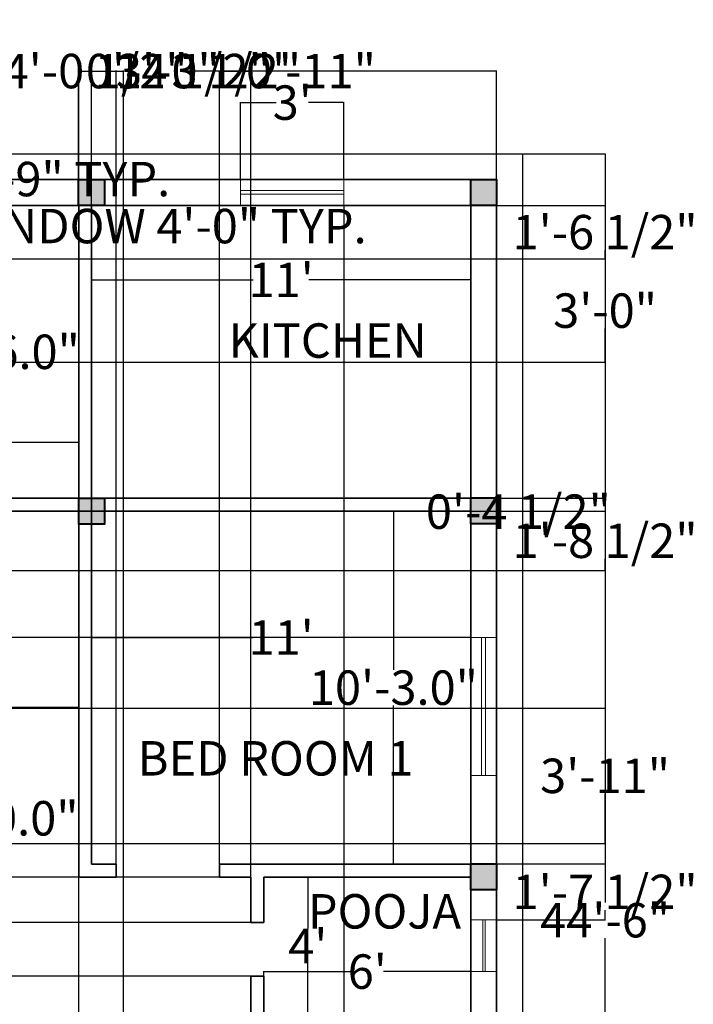
# Model space of a CAD drawing. Units: inches. Extents: x -132 to 363, y -548 to 79.
# Tile 3 of 3: x 128 to 363, y -264 to 79. Entities that reach past the tile are written whole.
import ezdxf

# ---------------------------------------------------------------- set-up
doc = ezdxf.new("R2010")
doc.units = ezdxf.units.IN
doc.header["$MEASUREMENT"] = 0
for name, color, linetype, lineweight in [('A-ANNO-DIMS', 2, 'Continuous', 18), ('A-AREA-IDEN', 7, 'Continuous', 25), ('A-COLS', 7, 'Continuous', 40), ('A-COLS-PATT', 252, 'Continuous', 13), ('A-GLAZ', 4, 'Continuous', 18), ('A-WALL', 7, 'Continuous', 35), ('C-PROP', 8, 'Continuous', 25)]:
    doc.layers.add(name, color=color, linetype=linetype, lineweight=lineweight)
doc.styles.get("Standard").update_dxf_attribs({"font": 'arial.ttf'})
doc.dimstyles.get("Standard").update_dxf_attribs({"dimtxt": 12, "dimasz": 0.18, "dimexe": 0.18, "dimexo": 0.0625, "dimgap": 0.09, "dimtad": 0, "dimtih": 1, "dimtoh": 1, "dimdec": 1, "dimzin": 0, "dimdsep": 46, "dimlunit": 3, "dimtxsty": 'Standard', "dimcen": 0.09, "dimadec": 0, "dimazin": 0, "dimtfac": 1, "dimtdec": 1, "dimtofl": 0, "dimtmove": 0, "dimatfit": 3, "dimfxl": 1, "dimtolj": 1, "dimtzin": 0, "dimarcsym": 0})

# ---------------------------------------------------------------- blocks, each defined once
blk = doc.blocks.new('*D1')
at = {"layer": 'A-ANNO-DIMS', "color": 0, "lineweight": -2, "transparency": 16777216}
for p, q in [((14.42, -87.55), (14.42, -68.07)), ((14.6, -68.25), (54.36, -68.25)), ((148.38, -68.25), (108.61, -68.25)), ((148.56, -87.55), (148.56, -68.07))]:
    blk.add_line(p, q, dxfattribs=at)
at = {"layer": 'A-ANNO-DIMS', "color": 0, "transparency": 16777216}
for points in [[(14.6, -68.22), (14.6, -68.28), (14.42, -68.25)], [(148.38, -68.22), (148.38, -68.28), (148.56, -68.25)]]:
    blk.add_solid(points, dxfattribs=at)
at = {"layer": 'Defpoints', "color": 0, "transparency": 16777216}
for p in [(148.56, -68.25), (14.42, -87.61), (148.56, -87.61)]:
    blk.add_point(p, dxfattribs=at)
at = {"layer": 'A-ANNO-DIMS', "color": 0, "transparency": 16777216, "insert": (81.49, -68.25), "char_height": 12, "attachment_point": 5}
blk.add_mtext('\\A1;11\'-2.1"', dxfattribs=at)
blk = doc.blocks.new('*D2')
at = {"layer": 'A-ANNO-DIMS', "color": 0, "lineweight": -2, "transparency": 16777216}
for p, q in [((148.4, 14.39), (123.86, 14.39)), ((124.04, 14.21), (124.04, -30.39)), ((124.04, -87.43), (124.04, -42.82)), ((148.45, -87.61), (123.86, -87.61))]:
    blk.add_line(p, q, dxfattribs=at)
at = {"layer": 'A-ANNO-DIMS', "color": 0, "transparency": 16777216}
for points in [[(124.01, 14.21), (124.07, 14.21), (124.04, 14.39)], [(124.01, -87.43), (124.07, -87.43), (124.04, -87.61)]]:
    blk.add_solid(points, dxfattribs=at)
at = {"layer": 'Defpoints', "color": 0, "transparency": 16777216}
for p in [(124.04, 14.39), (148.46, 14.39), (148.52, -87.61)]:
    blk.add_point(p, dxfattribs=at)
at = {"layer": 'A-ANNO-DIMS', "color": 0, "transparency": 16777216, "insert": (124.04, -36.61), "char_height": 12, "attachment_point": 5}
blk.add_mtext('\\A1;8\'-6.0"', dxfattribs=at)
blk = doc.blocks.new('*D3')
at = {"layer": 'A-ANNO-DIMS', "color": 0, "lineweight": -2, "transparency": 16777216}
for p, q in [((153.02, 14.33), (153.02, -11.75)), ((285.02, 14.33), (285.02, -11.75)), ((153.2, -11.57), (209.31, -11.57)), ((284.84, -11.57), (228.72, -11.57))]:
    blk.add_line(p, q, dxfattribs=at)
at = {"layer": 'A-ANNO-DIMS', "color": 0, "transparency": 16777216}
for points in [[(153.2, -11.54), (153.2, -11.6), (153.02, -11.57)], [(284.84, -11.54), (284.84, -11.6), (285.02, -11.57)]]:
    blk.add_solid(points, dxfattribs=at)
at = {"layer": 'Defpoints', "color": 0, "transparency": 16777216}
for p in [(153.02, 14.39), (285.02, 14.39), (285.02, -11.57)]:
    blk.add_point(p, dxfattribs=at)
at = {"layer": 'A-ANNO-DIMS', "color": 0, "transparency": 16777216, "insert": (219.02, -11.57), "char_height": 12, "attachment_point": 5}
blk.add_mtext("\\A1;11'", dxfattribs=at)
blk = doc.blocks.new('*D4')
at = {"layer": 'A-ANNO-DIMS', "color": 0, "lineweight": -2, "transparency": 16777216}
for p, q in [((284.95, -92.11), (257.94, -92.11)), ((258.12, -92.29), (258.12, -147.39)), ((258.12, -214.93), (258.12, -159.83)), ((284.95, -215.11), (257.94, -215.11))]:
    blk.add_line(p, q, dxfattribs=at)
at = {"layer": 'A-ANNO-DIMS', "color": 0, "transparency": 16777216}
for points in [[(258.09, -92.29), (258.15, -92.29), (258.12, -92.11)], [(258.09, -214.93), (258.15, -214.93), (258.12, -215.11)]]:
    blk.add_solid(points, dxfattribs=at)
at = {"layer": 'Defpoints', "color": 0, "transparency": 16777216}
for p in [(285.02, -92.11), (258.12, -215.11), (285.02, -215.11)]:
    blk.add_point(p, dxfattribs=at)
at = {"layer": 'A-ANNO-DIMS', "color": 0, "transparency": 16777216, "insert": (258.12, -153.61), "char_height": 12, "attachment_point": 5}
blk.add_mtext('\\A1;10\'-3.0"', dxfattribs=at)
blk = doc.blocks.new('*D5')
at = {"layer": 'A-ANNO-DIMS', "color": 0, "lineweight": -2, "transparency": 16777216}
for p, q in [((153.02, -134.95), (153.02, -136.33)), ((153.2, -136.15), (209.31, -136.15)), ((284.84, -136.15), (228.72, -136.15)), ((285.02, -136.09), (285.02, -135.97))]:
    blk.add_line(p, q, dxfattribs=at)
at = {"layer": 'A-ANNO-DIMS', "color": 0, "transparency": 16777216}
for points in [[(153.2, -136.12), (153.2, -136.18), (153.02, -136.15)], [(284.84, -136.12), (284.84, -136.18), (285.02, -136.15)]]:
    blk.add_solid(points, dxfattribs=at)
at = {"layer": 'Defpoints', "color": 0, "transparency": 16777216}
for p in [(153.02, -134.89), (285.02, -136.15), (285.02, -136.15)]:
    blk.add_point(p, dxfattribs=at)
at = {"layer": 'A-ANNO-DIMS', "color": 0, "transparency": 16777216, "insert": (219.02, -136.15), "char_height": 12, "attachment_point": 5}
blk.add_mtext("\\A1;11'", dxfattribs=at)
blk = doc.blocks.new('*D6')
at = {"layer": 'A-ANNO-DIMS', "color": 0, "lineweight": -2, "transparency": 16777216}
for p, q in [((213.08, -219.61), (228.48, -219.61)), ((228.3, -219.79), (228.3, -237.52)), ((228.3, -267.43), (228.3, -249.7)), ((213.08, -267.61), (228.48, -267.61))]:
    blk.add_line(p, q, dxfattribs=at)
at = {"layer": 'A-ANNO-DIMS', "color": 0, "transparency": 16777216}
for points in [[(228.27, -219.79), (228.33, -219.79), (228.3, -219.61)], [(228.27, -267.43), (228.33, -267.43), (228.3, -267.61)]]:
    blk.add_solid(points, dxfattribs=at)
at = {"layer": 'Defpoints', "color": 0, "transparency": 16777216}
for p in [(213.02, -219.61), (213.02, -267.61), (228.3, -267.61)]:
    blk.add_point(p, dxfattribs=at)
at = {"layer": 'A-ANNO-DIMS', "color": 0, "transparency": 16777216, "insert": (228.3, -243.61), "char_height": 12, "attachment_point": 5}
blk.add_mtext("\\A1;4'", dxfattribs=at)
blk = doc.blocks.new('*D7')
at = {"layer": 'A-ANNO-DIMS', "color": 0, "lineweight": -2, "transparency": 16777216}
for p, q in [((213.02, -254.06), (213.02, -252.33)), ((213.2, -252.51), (243.37, -252.51)), ((284.84, -252.51), (254.66, -252.51)), ((285.02, -252.45), (285.02, -252.33))]:
    blk.add_line(p, q, dxfattribs=at)
at = {"layer": 'A-ANNO-DIMS', "color": 0, "transparency": 16777216}
for points in [[(213.2, -252.48), (213.2, -252.54), (213.02, -252.51)], [(284.84, -252.48), (284.84, -252.54), (285.02, -252.51)]]:
    blk.add_solid(points, dxfattribs=at)
at = {"layer": 'Defpoints', "color": 0, "transparency": 16777216}
for p in [(285.02, -252.51), (285.02, -252.51), (213.02, -254.12)]:
    blk.add_point(p, dxfattribs=at)
at = {"layer": 'A-ANNO-DIMS', "color": 0, "transparency": 16777216, "insert": (249.02, -252.51), "char_height": 12, "attachment_point": 5}
blk.add_mtext("\\A1;6'", dxfattribs=at)
blk = doc.blocks.new('*D15')
at = {"layer": 'A-ANNO-DIMS', "color": 0, "lineweight": -2, "transparency": 16777216}
for p, q in [((14.42, -160.68), (14.42, -160.33)), ((14.6, -160.51), (54.34, -160.51)), ((148.34, -160.51), (108.59, -160.51)), ((148.52, -160.68), (148.52, -160.33))]:
    blk.add_line(p, q, dxfattribs=at)
at = {"layer": 'A-ANNO-DIMS', "color": 0, "transparency": 16777216}
for points in [[(14.6, -160.48), (14.6, -160.54), (14.42, -160.51)], [(148.34, -160.48), (148.34, -160.54), (148.52, -160.51)]]:
    blk.add_solid(points, dxfattribs=at)
at = {"layer": 'Defpoints', "color": 0, "transparency": 16777216}
for p in [(14.42, -160.75), (148.52, -160.51), (148.52, -160.75)]:
    blk.add_point(p, dxfattribs=at)
at = {"layer": 'A-ANNO-DIMS', "color": 0, "transparency": 16777216, "insert": (81.47, -160.51), "char_height": 12, "attachment_point": 5}
blk.add_mtext('\\A1;11\'-2.1"', dxfattribs=at)
blk = doc.blocks.new('*D16')
at = {"layer": 'A-ANNO-DIMS', "color": 0, "lineweight": -2, "transparency": 16777216}
for p, q in [((148.45, -92.11), (114.32, -92.11)), ((114.5, -92.29), (114.5, -192.89)), ((114.5, -305.93), (114.5, -205.32)), ((148.45, -306.11), (114.32, -306.11))]:
    blk.add_line(p, q, dxfattribs=at)
at = {"layer": 'A-ANNO-DIMS', "color": 0, "transparency": 16777216}
for points in [[(114.47, -92.29), (114.53, -92.29), (114.5, -92.11)], [(114.47, -305.93), (114.53, -305.93), (114.5, -306.11)]]:
    blk.add_solid(points, dxfattribs=at)
at = {"layer": 'Defpoints', "color": 0, "transparency": 16777216}
for p in [(148.52, -92.11), (114.5, -306.11), (148.52, -306.11)]:
    blk.add_point(p, dxfattribs=at)
at = {"layer": 'A-ANNO-DIMS', "color": 0, "transparency": 16777216, "insert": (114.5, -199.11), "char_height": 12, "attachment_point": 5}
blk.add_mtext('\\A1;17\'-10.0"', dxfattribs=at)
blk = doc.blocks.new('*D18')
at = {"layer": 'A-ANNO-DIMS', "color": 0, "lineweight": -2, "transparency": 16777216}
for p, q in [((204.9, 23.45), (204.9, 50.38)), ((205.08, 50.2), (217.3, 50.2)), ((240.72, 50.2), (228.51, 50.2)), ((240.9, 23.45), (240.9, 50.38))]:
    blk.add_line(p, q, dxfattribs=at)
at = {"layer": 'A-ANNO-DIMS', "color": 0, "transparency": 16777216}
for points in [[(205.08, 50.23), (205.08, 50.17), (204.9, 50.2)], [(240.72, 50.23), (240.72, 50.17), (240.9, 50.2)]]:
    blk.add_solid(points, dxfattribs=at)
at = {"layer": 'Defpoints', "color": 0, "transparency": 16777216}
for p in [(240.9, 50.2), (204.9, 23.39), (240.9, 23.39)]:
    blk.add_point(p, dxfattribs=at)
at = {"layer": 'A-ANNO-DIMS', "color": 0, "transparency": 16777216, "insert": (222.9, 50.2), "char_height": 12, "attachment_point": 5}
blk.add_mtext("\\A1;3'", dxfattribs=at)
blk = doc.blocks.new('WIN-48IN')
for p, q in [((48, 9), (0, 9)), ((0, 9), (0, 0)), ((48, 0), (48, 9)), ((0, 5.12), (48, 5.12)), ((48, 5.12), (0, 5.12)), ((0, 3.8), (48, 3.8)), ((0, 0), (48, 0))]:
    blk.add_line(p, q)
blk = doc.blocks.new('WIN-18IN')
for p, q in [((18, 9), (0, 9)), ((0, 9), (0, 0)), ((18, 0), (18, 9)), ((0, 6), (0, 0)), ((18, 5.06), (0, 5.06)), ((18, 4.2), (0, 4.2)), ((18, 0), (18, 6)), ((0, 0), (18, 0)), ((0, 0), (18, 0)), ((0, 0), (18, 0))]:
    blk.add_line(p, q)
blk = doc.blocks.new('*D21')
at = {"layer": 'A-ANNO-DIMS', "color": 0, "lineweight": -2, "transparency": 16777216}
for p, q in [((51.75, 14.33), (51.75, 7.01)), ((99.75, 14.33), (99.75, 7.01)), ((51.93, 7.19), (99.57, 7.19)), ((99.75, 7.19), (99.93, 7.19))]:
    blk.add_line(p, q, dxfattribs=at)
at = {"layer": 'A-ANNO-DIMS', "color": 0, "transparency": 16777216}
for points in [[(51.93, 7.22), (51.93, 7.16), (51.75, 7.19)], [(99.57, 7.22), (99.57, 7.16), (99.75, 7.19)]]:
    blk.add_solid(points, dxfattribs=at)
at = {"layer": 'Defpoints', "color": 0, "transparency": 16777216}
for p in [(51.75, 14.39), (99.75, 14.39), (99.75, 7.19)]:
    blk.add_point(p, dxfattribs=at)
at = {"layer": 'A-ANNO-DIMS', "color": 0, "transparency": 16777216, "insert": (175.94, 7.19), "char_height": 12, "attachment_point": 5}
blk.add_mtext('\\A1;WINDOW 4\'-0" TYP.', dxfattribs=at)
blk = doc.blocks.new('*D22')
at = {"layer": 'A-ANNO-DIMS', "color": 0, "lineweight": -2, "transparency": 16777216}
for p, q in [((99.81, 23.39), (107.13, 23.39)), ((106.95, 23.39), (106.95, 23.57)), ((106.95, 23.57), (107.13, 23.57)), ((106.95, 14.57), (106.95, 23.21)), ((99.81, 14.39), (107.13, 14.39))]:
    blk.add_line(p, q, dxfattribs=at)
at = {"layer": 'A-ANNO-DIMS', "color": 0, "transparency": 16777216}
for points in [[(106.92, 23.21), (106.98, 23.21), (106.95, 23.39)], [(106.92, 14.57), (106.98, 14.57), (106.95, 14.39)]]:
    blk.add_solid(points, dxfattribs=at)
at = {"layer": 'Defpoints', "color": 0, "transparency": 16777216}
for p in [(99.75, 23.39), (106.95, 23.39), (99.75, 14.39)]:
    blk.add_point(p, dxfattribs=at)
at = {"layer": 'A-ANNO-DIMS', "color": 0, "transparency": 16777216, "insert": (143.79, 23.57), "char_height": 12, "attachment_point": 5}
blk.add_mtext('\\A1;0\'-9" TYP.', dxfattribs=at)
blk = doc.blocks.new('*D26')
at = {"layer": 'A-ANNO-DIMS', "color": 0, "lineweight": -2, "transparency": 16777216}
for p, q in [((303.08, 32.39), (332, 32.39)), ((331.82, 32.21), (331.82, -228.39)), ((331.82, -501.43), (331.82, -240.82)), ((303.08, -501.61), (332, -501.61))]:
    blk.add_line(p, q, dxfattribs=at)
at = {"layer": 'A-ANNO-DIMS', "color": 0, "transparency": 16777216}
for points in [[(331.79, 32.21), (331.85, 32.21), (331.82, 32.39)], [(331.79, -501.43), (331.85, -501.43), (331.82, -501.61)]]:
    blk.add_solid(points, dxfattribs=at)
at = {"layer": 'Defpoints', "color": 0, "transparency": 16777216}
for p in [(303.02, 32.39), (303.02, -501.61), (331.82, -501.61)]:
    blk.add_point(p, dxfattribs=at)
at = {"layer": 'A-ANNO-DIMS', "color": 0, "transparency": 16777216, "insert": (331.82, -234.61), "char_height": 12, "attachment_point": 5}
blk.add_mtext('\\A1;44\'-6"', dxfattribs=at)
blk = doc.blocks.new('*D27')
at = {"layer": 'A-ANNO-DIMS', "color": 0, "lineweight": -2, "transparency": 16777216}
for p, q in [((5.42, 23.45), (5.42, 61.37)), ((5.6, 61.19), (114.93, 61.19)), ((293.84, 61.19), (184.5, 61.19)), ((294.02, 23.45), (294.02, 61.37))]:
    blk.add_line(p, q, dxfattribs=at)
at = {"layer": 'A-ANNO-DIMS', "color": 0, "transparency": 16777216}
for points in [[(5.6, 61.22), (5.6, 61.16), (5.42, 61.19)], [(293.84, 61.22), (293.84, 61.16), (294.02, 61.19)]]:
    blk.add_solid(points, dxfattribs=at)
at = {"layer": 'Defpoints', "color": 0, "transparency": 16777216}
for p in [(294.02, 61.19), (5.42, 23.39), (294.02, 23.39)]:
    blk.add_point(p, dxfattribs=at)
at = {"layer": 'A-ANNO-DIMS', "color": 0, "transparency": 16777216, "insert": (149.72, 61.19), "char_height": 12, "attachment_point": 5}
blk.add_mtext('\\A1;24\'-0 1/2"', dxfattribs=at)
blk = doc.blocks.new('*D30')
at = {"layer": 'A-ANNO-DIMS', "color": 0, "lineweight": -2, "transparency": 16777216}
for p, q in [((240.9, 14.33), (240.9, -530.59)), ((285.02, 14.33), (285.02, -530.59)), ((241.08, -530.41), (246.92, -530.41)), ((284.84, -530.41), (278.99, -530.41))]:
    blk.add_line(p, q, dxfattribs=at)
at = {"layer": 'A-ANNO-DIMS', "color": 0, "transparency": 16777216}
for points in [[(241.08, -530.38), (241.08, -530.44), (240.9, -530.41)], [(284.84, -530.38), (284.84, -530.44), (285.02, -530.41)]]:
    blk.add_solid(points, dxfattribs=at)
at = {"layer": 'Defpoints', "color": 0, "transparency": 16777216}
for p in [(240.9, 14.39), (285.02, 14.39), (285.02, -530.41)]:
    blk.add_point(p, dxfattribs=at)
at = {"layer": 'A-ANNO-DIMS', "color": 0, "transparency": 16777216, "insert": (262.96, -530.41), "char_height": 12, "attachment_point": 5}
blk.add_mtext('\\A1;3\'-8"', dxfattribs=at)
blk = doc.blocks.new('*D31')
at = {"layer": 'A-ANNO-DIMS', "color": 0, "lineweight": -2, "transparency": 16777216}
for p, q in [((14.48, 14.39), (332, 14.39)), ((331.82, 14.21), (331.82, 11.36)), ((331.82, -4.08), (331.82, -1.23)), ((14.48, -4.26), (332, -4.26))]:
    blk.add_line(p, q, dxfattribs=at)
at = {"layer": 'A-ANNO-DIMS', "color": 0, "transparency": 16777216}
for points in [[(331.79, 14.21), (331.85, 14.21), (331.82, 14.39)], [(331.79, -4.08), (331.85, -4.08), (331.82, -4.26)]]:
    blk.add_solid(points, dxfattribs=at)
at = {"layer": 'Defpoints', "color": 0, "transparency": 16777216}
for p in [(14.42, 14.39), (14.42, -4.26), (331.82, -4.26)]:
    blk.add_point(p, dxfattribs=at)
at = {"layer": 'A-ANNO-DIMS', "color": 0, "transparency": 16777216, "insert": (331.82, 5.07), "char_height": 12, "attachment_point": 5}
blk.add_mtext('\\A1;1\'-6 1/2"', dxfattribs=at)
blk = doc.blocks.new('*D32')
at = {"layer": 'A-ANNO-DIMS', "color": 0, "lineweight": -2, "transparency": 16777216}
for p, q in [((14.48, -4.26), (332, -4.26)), ((331.82, -4.44), (331.82, -16.04)), ((331.82, -40.08), (331.82, -28.48)), ((14.48, -40.26), (332, -40.26))]:
    blk.add_line(p, q, dxfattribs=at)
at = {"layer": 'A-ANNO-DIMS', "color": 0, "transparency": 16777216}
for points in [[(331.79, -4.44), (331.85, -4.44), (331.82, -4.26)], [(331.79, -40.08), (331.85, -40.08), (331.82, -40.26)]]:
    blk.add_solid(points, dxfattribs=at)
at = {"layer": 'Defpoints', "color": 0, "transparency": 16777216}
for p in [(14.42, -4.26), (14.42, -40.26), (331.82, -40.26)]:
    blk.add_point(p, dxfattribs=at)
at = {"layer": 'A-ANNO-DIMS', "color": 0, "transparency": 16777216, "insert": (331.82, -22.26), "char_height": 12, "attachment_point": 5}
blk.add_mtext('\\A1;3\'-0"', dxfattribs=at)
blk = doc.blocks.new('*D33')
at = {"layer": 'A-ANNO-DIMS', "color": 0, "lineweight": -2, "transparency": 16777216}
for p, q in [((14.48, -92.11), (332, -92.11)), ((331.82, -92.29), (331.82, -96.13)), ((331.82, -112.57), (331.82, -108.72)), ((14.48, -112.75), (332, -112.75))]:
    blk.add_line(p, q, dxfattribs=at)
at = {"layer": 'A-ANNO-DIMS', "color": 0, "transparency": 16777216}
for points in [[(331.79, -92.29), (331.85, -92.29), (331.82, -92.11)], [(331.79, -112.57), (331.85, -112.57), (331.82, -112.75)]]:
    blk.add_solid(points, dxfattribs=at)
at = {"layer": 'Defpoints', "color": 0, "transparency": 16777216}
for p in [(14.42, -92.11), (14.42, -112.75), (331.82, -112.75)]:
    blk.add_point(p, dxfattribs=at)
at = {"layer": 'A-ANNO-DIMS', "color": 0, "transparency": 16777216, "insert": (331.82, -102.43), "char_height": 12, "attachment_point": 5}
blk.add_mtext('\\A1;1\'-8 1/2"', dxfattribs=at)
blk = doc.blocks.new('*D34')
at = {"layer": 'A-ANNO-DIMS', "color": 0, "lineweight": -2, "transparency": 16777216}
for p, q in [((14.48, -160.75), (332, -160.75)), ((331.82, -160.93), (331.82, -178.11)), ((331.82, -207.73), (331.82, -190.55)), ((14.48, -207.91), (332, -207.91))]:
    blk.add_line(p, q, dxfattribs=at)
at = {"layer": 'A-ANNO-DIMS', "color": 0, "transparency": 16777216}
for points in [[(331.79, -160.93), (331.85, -160.93), (331.82, -160.75)], [(331.79, -207.73), (331.85, -207.73), (331.82, -207.91)]]:
    blk.add_solid(points, dxfattribs=at)
at = {"layer": 'Defpoints', "color": 0, "transparency": 16777216}
for p in [(14.42, -160.75), (14.42, -207.91), (331.82, -207.91)]:
    blk.add_point(p, dxfattribs=at)
at = {"layer": 'A-ANNO-DIMS', "color": 0, "transparency": 16777216, "insert": (331.82, -184.33), "char_height": 12, "attachment_point": 5}
blk.add_mtext('\\A1;3\'-11"', dxfattribs=at)
blk = doc.blocks.new('*D35')
at = {"layer": 'A-ANNO-DIMS', "color": 0, "lineweight": -2, "transparency": 16777216}
for p, q in [((284.95, -92.11), (-70.46, -92.11)), ((-70.28, -92.29), (-70.28, -107.91)), ((-70.28, -135.97), (-70.28, -120.35)), ((284.95, -136.15), (-70.46, -136.15))]:
    blk.add_line(p, q, dxfattribs=at)
at = {"layer": 'A-ANNO-DIMS', "color": 0, "transparency": 16777216}
for points in [[(-70.31, -92.29), (-70.25, -92.29), (-70.28, -92.11)], [(-70.31, -135.97), (-70.25, -135.97), (-70.28, -136.15)]]:
    blk.add_solid(points, dxfattribs=at)
at = {"layer": 'Defpoints', "color": 0, "transparency": 16777216}
for p in [(285.02, -92.11), (-70.28, -136.15), (285.02, -136.15)]:
    blk.add_point(p, dxfattribs=at)
at = {"layer": 'A-ANNO-DIMS', "color": 0, "transparency": 16777216, "insert": (-70.28, -114.13), "char_height": 12, "attachment_point": 5}
blk.add_mtext('\\A1;3\'-8"', dxfattribs=at)
blk = doc.blocks.new('*D36')
at = {"layer": 'A-ANNO-DIMS', "color": 0, "lineweight": -2, "transparency": 16777216}
for p, q in [((294.08, -215.01), (332, -215.01)), ((331.82, -215.19), (331.82, -218.47)), ((331.82, -234.33), (331.82, -231.06)), ((294.08, -234.51), (332, -234.51))]:
    blk.add_line(p, q, dxfattribs=at)
at = {"layer": 'A-ANNO-DIMS', "color": 0, "transparency": 16777216}
for points in [[(331.79, -215.19), (331.85, -215.19), (331.82, -215.01)], [(331.79, -234.33), (331.85, -234.33), (331.82, -234.51)]]:
    blk.add_solid(points, dxfattribs=at)
at = {"layer": 'Defpoints', "color": 0, "transparency": 16777216}
for p in [(294.02, -215.01), (294.02, -234.51), (331.82, -234.51)]:
    blk.add_point(p, dxfattribs=at)
at = {"layer": 'A-ANNO-DIMS', "color": 0, "transparency": 16777216, "insert": (331.82, -224.76), "char_height": 12, "attachment_point": 5}
blk.add_mtext('\\A1;1\'-7 1/2"', dxfattribs=at)
blk = doc.blocks.new('*D44')
at = {"layer": 'A-ANNO-DIMS', "color": 0, "lineweight": -2, "transparency": 16777216}
for p, q in [((161.59, -215.05), (161.59, 61.37)), ((161.77, 61.19), (163.55, 61.19)), ((197.41, 61.19), (195.62, 61.19)), ((197.59, -215.05), (197.59, 61.37))]:
    blk.add_line(p, q, dxfattribs=at)
at = {"layer": 'A-ANNO-DIMS', "color": 0, "transparency": 16777216}
for points in [[(161.77, 61.22), (161.77, 61.16), (161.59, 61.19)], [(197.41, 61.22), (197.41, 61.16), (197.59, 61.19)]]:
    blk.add_solid(points, dxfattribs=at)
at = {"layer": 'Defpoints', "color": 0, "transparency": 16777216}
for p in [(197.59, 61.19), (161.59, -215.11), (197.59, -215.11)]:
    blk.add_point(p, dxfattribs=at)
at = {"layer": 'A-ANNO-DIMS', "color": 0, "transparency": 16777216, "insert": (179.59, 61.19), "char_height": 12, "attachment_point": 5}
blk.add_mtext('\\A1;3\'-0"', dxfattribs=at)
blk = doc.blocks.new('*D46')
at = {"layer": 'A-ANNO-DIMS', "color": 0, "lineweight": -2, "transparency": 16777216}
for p, q in [((208.45, -235.36), (-70.46, -235.36)), ((-70.28, -235.54), (-70.28, -238.62)), ((-70.28, -253.94), (-70.28, -250.85)), ((208.45, -254.12), (-70.46, -254.12))]:
    blk.add_line(p, q, dxfattribs=at)
at = {"layer": 'A-ANNO-DIMS', "color": 0, "transparency": 16777216}
for points in [[(-70.31, -235.54), (-70.25, -235.54), (-70.28, -235.36)], [(-70.31, -253.94), (-70.25, -253.94), (-70.28, -254.12)]]:
    blk.add_solid(points, dxfattribs=at)
at = {"layer": 'Defpoints', "color": 0, "transparency": 16777216}
for p in [(208.52, -235.36), (-70.28, -254.12), (208.52, -254.12)]:
    blk.add_point(p, dxfattribs=at)
at = {"layer": 'A-ANNO-DIMS', "color": 0, "transparency": 16777216, "insert": (-70.28, -244.74), "char_height": 12, "attachment_point": 5}
blk.add_mtext('\\A1;1\'-7"', dxfattribs=at)
blk = doc.blocks.new('*D48')
at = {"layer": 'A-ANNO-DIMS', "color": 0, "lineweight": -2, "transparency": 16777216}
for p, q in [((197.59, -219.55), (197.59, 61.37)), ((197.77, 61.19), (208.34, 61.19)), ((208.52, -219.55), (208.52, 61.37)), ((208.52, 61.19), (208.7, 61.19))]:
    blk.add_line(p, q, dxfattribs=at)
at = {"layer": 'A-ANNO-DIMS', "color": 0, "transparency": 16777216}
for points in [[(197.77, 61.22), (197.77, 61.16), (197.59, 61.19)], [(208.34, 61.22), (208.34, 61.16), (208.52, 61.19)]]:
    blk.add_solid(points, dxfattribs=at)
at = {"layer": 'Defpoints', "color": 0, "transparency": 16777216}
for p in [(208.52, 61.19), (197.59, -219.61), (208.52, -219.61)]:
    blk.add_point(p, dxfattribs=at)
at = {"layer": 'A-ANNO-DIMS', "color": 0, "transparency": 16777216, "insert": (229.4, 61.19), "char_height": 12, "attachment_point": 5}
blk.add_mtext('\\A1;0\'-11"', dxfattribs=at)
blk = doc.blocks.new('*D50')
at = {"layer": 'A-ANNO-DIMS', "color": 0, "lineweight": -2, "transparency": 16777216}
for p, q in [((208.45, -219.61), (-70.46, -219.61)), ((-70.28, -219.79), (-70.28, -221.37)), ((208.45, -235.36), (-70.46, -235.36)), ((-70.28, -235.18), (-70.28, -233.6))]:
    blk.add_line(p, q, dxfattribs=at)
at = {"layer": 'A-ANNO-DIMS', "color": 0, "transparency": 16777216}
for points in [[(-70.31, -219.79), (-70.25, -219.79), (-70.28, -219.61)], [(-70.31, -235.18), (-70.25, -235.18), (-70.28, -235.36)]]:
    blk.add_solid(points, dxfattribs=at)
at = {"layer": 'Defpoints', "color": 0, "transparency": 16777216}
for p in [(208.52, -219.61), (-70.28, -235.36), (208.52, -235.36)]:
    blk.add_point(p, dxfattribs=at)
at = {"layer": 'A-ANNO-DIMS', "color": 0, "transparency": 16777216, "insert": (-70.28, -227.48), "char_height": 12, "attachment_point": 5}
blk.add_mtext('\\A1;1\'-4"', dxfattribs=at)
blk = doc.blocks.new('*D52')
at = {"layer": 'A-ANNO-DIMS', "color": 0, "lineweight": -2, "transparency": 16777216}
for p, q in [((148.46, 14.45), (148.46, 61.37)), ((148.64, 61.19), (152.84, 61.19)), ((153.02, 14.45), (153.02, 61.37)), ((153.02, 61.19), (153.2, 61.19))]:
    blk.add_line(p, q, dxfattribs=at)
at = {"layer": 'A-ANNO-DIMS', "color": 0, "transparency": 16777216}
for points in [[(148.64, 61.22), (148.64, 61.16), (148.46, 61.19)], [(152.84, 61.22), (152.84, 61.16), (153.02, 61.19)]]:
    blk.add_solid(points, dxfattribs=at)
at = {"layer": 'Defpoints', "color": 0, "transparency": 16777216}
for p in [(153.02, 61.19), (148.46, 14.39), (153.02, 14.39)]:
    blk.add_point(p, dxfattribs=at)
at = {"layer": 'A-ANNO-DIMS', "color": 0, "transparency": 16777216, "insert": (183.22, 61.19), "char_height": 12, "attachment_point": 5}
blk.add_mtext('\\A1;0\'-4 1/2"', dxfattribs=at)
blk = doc.blocks.new('*D57')
at = {"layer": 'A-ANNO-DIMS', "color": 0, "lineweight": -2, "transparency": 16777216}
for p, q in [((148.52, -267.55), (148.52, 61.37)), ((148.7, 61.19), (163.91, 61.19)), ((164.09, -267.55), (164.09, 61.37)), ((164.09, 61.19), (164.27, 61.19))]:
    blk.add_line(p, q, dxfattribs=at)
at = {"layer": 'A-ANNO-DIMS', "color": 0, "transparency": 16777216}
for points in [[(148.7, 61.22), (148.7, 61.16), (148.52, 61.19)], [(163.91, 61.22), (163.91, 61.16), (164.09, 61.19)]]:
    blk.add_solid(points, dxfattribs=at)
at = {"layer": 'Defpoints', "color": 0, "transparency": 16777216}
for p in [(164.09, 61.19), (148.52, -267.61), (164.09, -267.61)]:
    blk.add_point(p, dxfattribs=at)
at = {"layer": 'A-ANNO-DIMS', "color": 0, "transparency": 16777216, "insert": (193.73, 61.19), "char_height": 12, "attachment_point": 5}
blk.add_mtext('\\A1;1\'-3 1/2"', dxfattribs=at)
blk = doc.blocks.new('*D58')
at = {"layer": 'A-ANNO-DIMS', "color": 0, "lineweight": -2, "transparency": 16777216}
for p, q in [((285.08, -87.61), (332, -87.61)), ((331.82, -87.79), (331.82, -91.93)), ((285.08, -92.11), (332, -92.11)), ((331.82, -92.29), (331.64, -92.29)), ((331.82, -92.11), (331.82, -92.29))]:
    blk.add_line(p, q, dxfattribs=at)
at = {"layer": 'A-ANNO-DIMS', "color": 0, "transparency": 16777216}
for points in [[(331.79, -87.79), (331.85, -87.79), (331.82, -87.61)], [(331.79, -91.93), (331.85, -91.93), (331.82, -92.11)]]:
    blk.add_solid(points, dxfattribs=at)
at = {"layer": 'Defpoints', "color": 0, "transparency": 16777216}
for p in [(285.02, -87.61), (285.02, -92.11), (331.82, -92.11)]:
    blk.add_point(p, dxfattribs=at)
at = {"layer": 'A-ANNO-DIMS', "color": 0, "transparency": 16777216, "insert": (301.62, -92.29), "char_height": 12, "attachment_point": 5}
blk.add_mtext('\\A1;0\'-4 1/2"', dxfattribs=at)

msp = doc.modelspace()

# ---------------------------------------------------------------- hatches: boundary and pattern name
at = {"layer": 'A-COLS-PATT'}
h = msp.add_hatch(color=256, dxfattribs=at)
h.dxf.hatch_style = 1
h.paths.add_polyline_path([(14.42, 23.39), (6.02, 23.39), (5.42, 23.39), (5.42, 14.39), (14.42, 14.39)])
h.paths.add_polyline_path([(14.42, -87.61), (5.42, -87.61), (5.42, -96.61), (14.42, -96.61)])
h.paths.add_polyline_path([(153.02, -87.61), (148.56, -87.61), (148.56, -96.61), (153.02, -96.61)])
h.paths.add_polyline_path([(157.56, -87.61), (153.02, -87.61), (153.02, -92.11), (157.56, -92.11)])
h.paths.add_polyline_path([(157.56, -92.11), (153.02, -92.11), (153.02, -96.61), (157.56, -96.61)])
h.paths.add_polyline_path([(294.02, -87.49), (285.02, -87.49), (285.02, -96.49), (294.02, -96.49)])
h.paths.add_polyline_path([(294.02, -215.01), (285.02, -215.01), (285.02, -224.01), (294.02, -224.01)])
h.paths.add_polyline_path([(294.02, -267.43), (285.02, -267.43), (285.02, -277.01), (294.02, -277.01)])
h.paths.add_polyline_path([(294.02, -406.11), (285.02, -406.11), (285.02, -415.11), (294.02, -415.11)])
h.paths.add_polyline_path([(161.71, -406.11), (148.52, -406.11), (148.52, -415.11), (161.71, -415.11)])
h.paths.add_polyline_path([(157.51, -267.61), (148.52, -267.61), (148.52, -276.61), (157.51, -276.61)])
h.paths.add_polyline_path([(14.42, -268.43), (5.42, -268.43), (5.42, -277.43), (14.42, -277.43)])
h = msp.add_hatch(color=256, dxfattribs=at)
h.dxf.hatch_style = 1
h.paths.add_polyline_path([(294.02, 23.39), (285.02, 23.39), (285.02, 14.39), (294.02, 14.39)])
h.paths.add_polyline_path([(157.46, 23.39), (148.46, 23.39), (148.46, 14.39), (157.46, 14.39)])
h = msp.add_hatch(color=256, dxfattribs=at)
h.dxf.hatch_style = 1
h.paths.add_polyline_path([(285.02, 23.39), (285.02, 14.39), (294.02, 14.39), (294.02, 23.39)])
h.paths.add_polyline_path([(148.46, 23.39), (148.46, 14.39), (157.46, 14.39), (157.46, 23.39)])

# ---------------------------------------------------------------- linework, layer by layer
at = {"layer": 'A-COLS'}
for points in [[(148.46, 23.39), (157.46, 23.39), (157.46, 14.39), (148.46, 14.39)], [(285.02, 23.39), (294.02, 23.39), (294.02, 14.39), (285.02, 14.39)], [(148.56, -87.61), (157.56, -87.61), (157.56, -96.61), (148.56, -96.61)], [(285.02, -87.49), (294.02, -87.49), (294.02, -96.49), (285.02, -96.49)], [(285.02, -215.01), (294.02, -215.01), (294.02, -224.01), (285.02, -224.01)]]:
    msp.add_lwpolyline(points, close=True, dxfattribs=at)
at = {"layer": 'A-GLAZ'}
for p, q in [((240.9, 23.39), (204.9, 23.39)), ((204.9, 23.39), (204.9, 14.39)), ((240.9, 14.39), (240.9, 23.39)), ((240.9, 19.59), (204.9, 19.59)), ((240.9, 18.28), (204.9, 18.28)), ((204.9, 18.28), (240.9, 18.28)), ((204.9, 14.39), (240.9, 14.39)), ((204.9, 14.39), (240.9, 14.39))]:
    msp.add_line(p, q, dxfattribs=at)
at = {"layer": 'A-WALL'}
for p, q in [((6.02, 23.39), (294.02, 23.39)), ((294.02, 23.39), (294.02, -492.61)), ((14.42, 14.39), (285.02, 14.39)), ((148.52, 14.39), (148.52, -219.61)), ((153.02, 14.39), (153.02, -215.11)), ((285.02, 14.39), (285.02, -492.61)), ((14.42, -87.61), (148.52, -87.61)), ((153.02, -87.61), (285.02, -87.61)), ((14.42, -92.11), (148.52, -92.11)), ((153.02, -92.11), (285.02, -92.11)), ((153.02, -215.11), (161.59, -215.11)), ((161.59, -215.11), (161.59, -219.61)), ((197.59, -219.61), (197.59, -215.11)), ((197.59, -215.11), (285.02, -215.11)), ((148.52, -219.61), (161.59, -219.61)), ((197.59, -219.61), (208.52, -219.61)), ((208.52, -219.61), (208.52, -235.36)), ((213.02, -219.61), (213.02, -235.36)), ((213.02, -219.61), (285.02, -219.61)), ((213.02, -235.36), (208.52, -235.36)), ((208.52, -254.12), (213.02, -254.12)), ((208.52, -254.12), (208.52, -267.61)), ((213.02, -254.12), (213.02, -267.61))]:
    msp.add_line(p, q, dxfattribs=at)
at = {"layer": 'C-PROP'}
for p, q in [((6.02, 32.39), (294.02, 32.39)), ((294.02, 32.39), (303.02, 32.39)), ((303.02, 32.39), (303.02, -501.61))]:
    msp.add_line(p, q, dxfattribs=at)

# ---------------------------------------------------------------- block references
at = {"layer": 'A-GLAZ'}
for name, p, rotation in [('WIN-48IN', (285.02, -136.15), 269.9999999999999), ('WIN-18IN', (285.02, -234.51), 270.000000000001)]:
    msp.add_blockref(name, p, dxfattribs=dict(at, rotation=rotation))

# ---------------------------------------------------------------- texts
at = {"layer": 'A-AREA-IDEN'}
for s, p in [('KITCHEN', (200.7, -38.69)), ('BED ROOM 1', (169.05, -184.22)), ('POOJA', (228.3, -237.52))]:
    msp.add_text(s, height=12, dxfattribs=at).set_placement(p)

# ---------------------------------------------------------------- dimensions: what is measured, and where the dimension line sits
at = {"layer": 'A-ANNO-DIMS'}
for base, p1, p2, override, picture, middle in [((294.02, 61.19), (5.42, 23.39), (294.02, 23.39), {"dimdec": 1, "dimlfac": 1, "dimrnd": 0, "dimzin": 1, "dimdsep": 46, "dimlunit": 4, "dimfrac": 2}, '*D27', (149.72, 61.19)), ((153.02, 61.19), (148.46, 14.39), (153.02, 14.39), {"dimdec": 1, "dimlfac": 1, "dimrnd": 0, "dimzin": 1, "dimdsep": 46, "dimlunit": 4, "dimfrac": 2}, '*D52', (183.22, 61.19)), ((164.09, 61.19), (148.52, -267.61), (164.09, -267.61), {"dimdec": 1, "dimlfac": 1, "dimrnd": 0, "dimzin": 1, "dimdsep": 46, "dimlunit": 4, "dimfrac": 2}, '*D57', (193.73, 61.19)), ((197.59, 61.19), (161.59, -215.11), (197.59, -215.11), {"dimdec": 1, "dimlfac": 1, "dimrnd": 0, "dimzin": 1, "dimdsep": 46, "dimlunit": 4, "dimfrac": 2}, '*D44', (179.59, 61.19)), ((208.52, 61.19), (197.59, -219.61), (208.52, -219.61), {"dimdec": 1, "dimlfac": 1, "dimrnd": 0, "dimzin": 1, "dimdsep": 46, "dimlunit": 4, "dimfrac": 2}, '*D48', (229.4, 61.19)), ((240.9, 50.2), (204.9, 23.39), (240.9, 23.39), {"dimclrd": 0, "dimclre": 0, "dimclrt": 0}, '*D18', (222.9, 50.2)), ((285.02, -11.57), (153.02, 14.39), (285.02, 14.39), {"dimclrd": 0, "dimclre": 0, "dimclrt": 0}, '*D3', (219.02, -11.57)), ((285.02, -530.41), (240.9, 14.39), (285.02, 14.39), {"dimdec": 1, "dimlfac": 1, "dimrnd": 0, "dimzin": 1, "dimdsep": 46, "dimlunit": 4, "dimfrac": 2}, '*D30', (262.96, -530.41)), ((148.56, -68.25), (14.42, -87.61), (148.56, -87.61), {"dimclrd": 0, "dimclre": 0, "dimclrt": 0}, '*D1', (81.49, -68.25)), ((285.02, -136.15), (153.02, -134.89), (285.02, -136.15), {"dimclrd": 0, "dimclre": 0, "dimclrt": 0}, '*D5', (219.02, -136.15)), ((148.52, -160.51), (14.42, -160.75), (148.52, -160.75), {"dimclrd": 0, "dimclre": 0, "dimclrt": 0}, '*D15', (81.47, -160.51)), ((285.02, -252.51), (213.02, -254.12), (285.02, -252.51), {"dimclrd": 0, "dimclre": 0, "dimclrt": 0}, '*D7', (249.02, -252.51))]:
    dim = msp.add_linear_dim(base=base, p1=p1, p2=p2, dimstyle='Standard', override=override, dxfattribs=at)
    dim.commit()
    dim.dimension.update_dxf_attribs({"geometry": picture, "text_midpoint": middle})
dim = msp.add_linear_dim(base=(106.95, 23.39), p1=(99.75, 14.39), p2=(99.75, 23.39), angle=90, text='<> TYP.', dimstyle='Standard', override={"dimdec": 1, "dimlfac": 1, "dimrnd": 0, "dimzin": 1, "dimdsep": 46, "dimlunit": 4, "dimfrac": 2}, dxfattribs=at)
dim.commit()
dim.dimension.update_dxf_attribs({"geometry": '*D22', "text_midpoint": (143.79, 23.57)})
dim = msp.add_linear_dim(base=(99.75, 7.19), p1=(51.75, 14.39), p2=(99.75, 14.39), text='WINDOW <> TYP.', dimstyle='Standard', override={"dimdec": 1, "dimlfac": 1, "dimrnd": 0, "dimzin": 1, "dimdsep": 46, "dimlunit": 4, "dimfrac": 2}, dxfattribs=at)
dim.commit()
dim.dimension.update_dxf_attribs({"geometry": '*D21', "text_midpoint": (175.94, 7.19)})
for base, p1, p2, override, picture, middle in [((331.82, -501.61), (303.02, 32.39), (303.02, -501.61), {"dimdec": 1, "dimlfac": 1, "dimrnd": 0, "dimzin": 1, "dimdsep": 46, "dimlunit": 4, "dimfrac": 2}, '*D26', (331.82, -234.61)), ((331.8158, -4.2561), (14.4158, 14.392), (14.4158, -4.2561), {"dimdec": 1, "dimlfac": 1, "dimrnd": 0, "dimzin": 1, "dimdsep": 46, "dimlunit": 4, "dimfrac": 2}, '*D31', (331.8158, 5.068)), ((124.04, 14.39), (148.52, -87.61), (148.46, 14.39), {"dimclrd": 0, "dimclre": 0, "dimclrt": 0}, '*D2', (124.04, -36.61)), ((331.82, -40.26), (14.42, -4.26), (14.42, -40.26), {"dimdec": 1, "dimlfac": 1, "dimrnd": 0, "dimzin": 1, "dimdsep": 46, "dimlunit": 4, "dimfrac": 2}, '*D32', (331.82, -22.26)), ((331.82, -92.11), (285.02, -87.61), (285.02, -92.11), {"dimdec": 1, "dimlfac": 1, "dimrnd": 0, "dimzin": 1, "dimdsep": 46, "dimlunit": 4, "dimfrac": 2}, '*D58', (301.62, -92.29)), ((331.82, -112.75), (14.42, -92.11), (14.42, -112.75), {"dimdec": 1, "dimlfac": 1, "dimrnd": 0, "dimzin": 1, "dimdsep": 46, "dimlunit": 4, "dimfrac": 2}, '*D33', (331.82, -102.43)), ((-70.28, -136.15), (285.02, -92.11), (285.02, -136.15), {"dimdec": 1, "dimlfac": 1, "dimrnd": 0, "dimzin": 1, "dimdsep": 46, "dimlunit": 4, "dimfrac": 2}, '*D35', (-70.28, -114.13)), ((114.5, -306.11), (148.52, -92.11), (148.52, -306.11), {"dimclrd": 0, "dimclre": 0, "dimclrt": 0}, '*D16', (114.5, -199.11)), ((258.12, -215.11), (285.02, -92.11), (285.02, -215.11), {"dimclrd": 0, "dimclre": 0, "dimclrt": 0}, '*D4', (258.12, -153.61)), ((331.82, -207.91), (14.42, -160.75), (14.42, -207.91), {"dimdec": 1, "dimlfac": 1, "dimrnd": 0, "dimzin": 1, "dimdsep": 46, "dimlunit": 4, "dimfrac": 2}, '*D34', (331.82, -184.33)), ((331.82, -234.51), (294.02, -215.01), (294.02, -234.51), {"dimdec": 1, "dimlfac": 1, "dimrnd": 0, "dimzin": 1, "dimdsep": 46, "dimlunit": 4, "dimfrac": 2}, '*D36', (331.82, -224.76)), ((-70.2842, -235.3581), (208.5158, -219.608), (208.5158, -235.3581), {"dimdec": 1, "dimlfac": 1, "dimrnd": 0, "dimzin": 1, "dimdsep": 46, "dimlunit": 4, "dimfrac": 2}, '*D50', (-70.2842, -227.483)), ((228.3, -267.61), (213.02, -219.61), (213.02, -267.61), {"dimclrd": 0, "dimclre": 0, "dimclrt": 0}, '*D6', (228.3, -243.61)), ((-70.28, -254.12), (208.52, -235.36), (208.52, -254.12), {"dimdec": 1, "dimlfac": 1, "dimrnd": 0, "dimzin": 1, "dimdsep": 46, "dimlunit": 4, "dimfrac": 2}, '*D46', (-70.28, -244.74))]:
    dim = msp.add_linear_dim(base=base, p1=p1, p2=p2, angle=90, dimstyle='Standard', override=override, dxfattribs=at)
    dim.commit()
    dim.dimension.update_dxf_attribs({"geometry": picture, "text_midpoint": middle})

doc.saveas('drawing.dxf')
